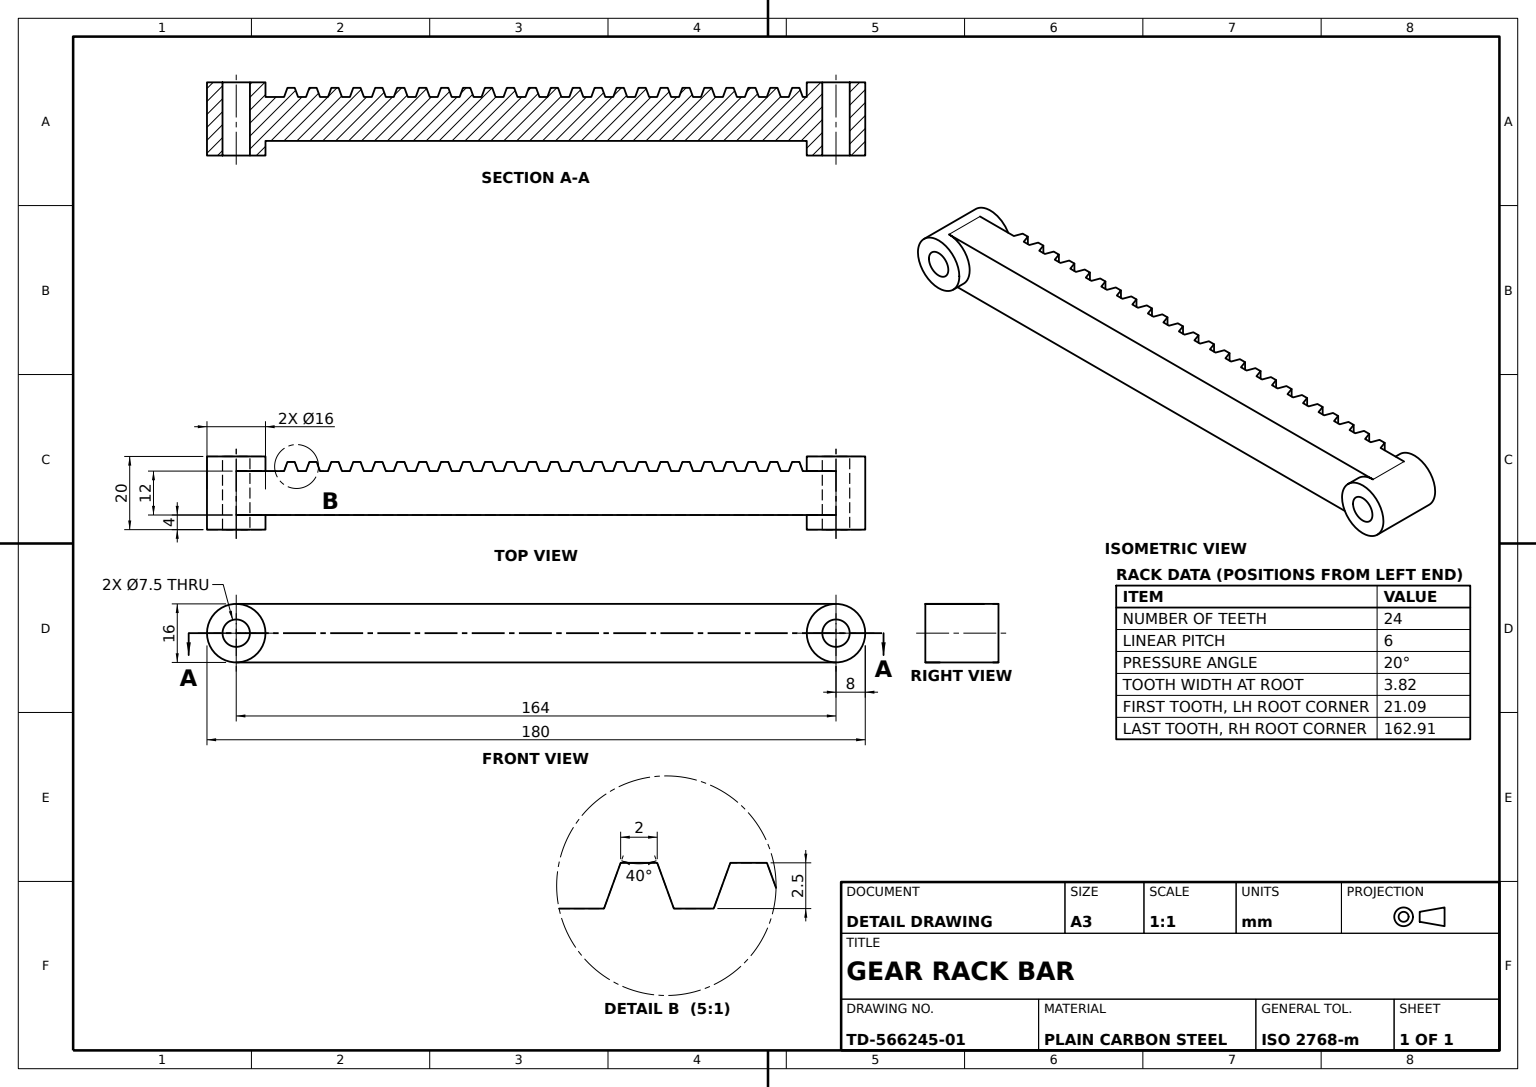
SolidWorks part; units mm, degrees
material "Plain Carbon Steel"
ref_plane "Front Plane" through (0, 0, 0) normal (0, 0, 1) x (1, 0, 0)
ref_plane "Top Plane" through (0, 0, 0) normal (0, 1, 0) x (1, 0, 0)
ref_plane "Right Plane" through (0, 0, 0) normal (1, 0, 0) x (0, 0, -1)
sketch "Eye Bar Profile Sketch" plane through (0, 0, 0) normal (1, 0, 0) x (0, 0, -1)
  circle A0 centre (0, 0) radius 8
  circle A1 centre (0, 0) radius 3.75
  circle A2 centre (-164, 0) radius 8
  circle A3 centre (-164, 0) radius 3.75
  dimension "D1" = 7.5
  dimension "D2" = 7.5
  dimension "D3" = 16
  dimension "D4" = 16
  dimension "D5" = 164
extrude "Bar With Eye Ends" add sketch "Eye Bar Profile Sketch" along normal mid plane 20
sketch "Rack Body Sketch" plane through (0, 0, 0) normal (1, 0, 0) x (0, 0, -1)
  line L1 (-164, 8) -> (0, 8)
  line L3 (-164, -8) -> (0, -8)
  circle A0 centre (-164, 0) radius 8 construction
  circle A1 centre (0, 0) radius 8 construction
  arc A2 (-164, -8) -> (-164, 8) centre (-164, 0) ccw
  circle A3 centre (0, 0) radius 8
  arc A4 (0, 8) -> (0, -8) centre (0, 0) ccw
  dimension "D1" = 0
extrude "Rack Body" add sketch "Rack Body Sketch" along normal mid plane 12
sketch "Rack Teeth Profile Sketch" plane through (0, 0, 0) normal (0, 1, 0) x (1, 0, 0)
  line L0 (0, 0) -> (-8.5, 0) construction
  line L1 (-10, 8) -> (-10, -10) construction
  line L2 (-8.5, 0) -> (-8.5, -10) construction
  line L3 (-8.5, -10) -> (-8.5, -12)
  line L4 (-8.5, -11) -> (-6, -11) construction
  line L5 (-6, 0) -> (-6, -164) construction
  line L6 (-8.5, -10) -> (-5.4907, -8.9047)
  line L7 (-8.5, -12) -> (-5.4907, -13.0953)
  line L8 (-5.4907, -8.9047) -> (-5.4907, -13.0953)
  line L9 (-8.5, -16) -> (-5.4907, -14.9047)
  line L10 (-5.4907, -14.9047) -> (-5.4907, -19.0953)
  line L11 (-8.5, -18) -> (-5.4907, -19.0953)
  line L12 (-8.5, -16) -> (-8.5, -18)
  line L13 (-8.5, -22) -> (-5.4907, -20.9047)
  line L14 (-5.4907, -20.9047) -> (-5.4907, -25.0953)
  line L15 (-8.5, -24) -> (-5.4907, -25.0953)
  line L16 (-8.5, -22) -> (-8.5, -24)
  line L17 (-8.5, -28) -> (-5.4907, -26.9047)
  line L18 (-5.4907, -26.9047) -> (-5.4907, -31.0953)
  line L19 (-8.5, -30) -> (-5.4907, -31.0953)
  line L20 (-8.5, -28) -> (-8.5, -30)
  line L21 (-8.5, -34) -> (-5.4907, -32.9047)
  line L22 (-5.4907, -32.9047) -> (-5.4907, -37.0953)
  line L23 (-8.5, -36) -> (-5.4907, -37.0953)
  line L24 (-8.5, -34) -> (-8.5, -36)
  line L25 (-8.5, -40) -> (-5.4907, -38.9047)
  line L26 (-5.4907, -38.9047) -> (-5.4907, -43.0953)
  line L27 (-8.5, -42) -> (-5.4907, -43.0953)
  line L28 (-8.5, -40) -> (-8.5, -42)
  line L29 (-8.5, -46) -> (-5.4907, -44.9047)
  line L30 (-5.4907, -44.9047) -> (-5.4907, -49.0953)
  line L31 (-8.5, -48) -> (-5.4907, -49.0953)
  line L32 (-8.5, -46) -> (-8.5, -48)
  line L33 (-8.5, -52) -> (-5.4907, -50.9047)
  line L34 (-5.4907, -50.9047) -> (-5.4907, -55.0953)
  line L35 (-8.5, -54) -> (-5.4907, -55.0953)
  line L36 (-8.5, -52) -> (-8.5, -54)
  line L37 (-8.5, -58) -> (-5.4907, -56.9047)
  line L38 (-5.4907, -56.9047) -> (-5.4907, -61.0953)
  line L39 (-8.5, -60) -> (-5.4907, -61.0953)
  line L40 (-8.5, -58) -> (-8.5, -60)
  line L41 (-8.5, -64) -> (-5.4907, -62.9047)
  line L42 (-5.4907, -62.9047) -> (-5.4907, -67.0953)
  line L43 (-8.5, -66) -> (-5.4907, -67.0953)
  line L44 (-8.5, -64) -> (-8.5, -66)
  line L45 (-8.5, -70) -> (-5.4907, -68.9047)
  line L46 (-5.4907, -68.9047) -> (-5.4907, -73.0953)
  line L47 (-8.5, -72) -> (-5.4907, -73.0953)
  line L48 (-8.5, -70) -> (-8.5, -72)
  line L49 (-8.5, -76) -> (-5.4907, -74.9047)
  line L50 (-5.4907, -74.9047) -> (-5.4907, -79.0953)
  line L51 (-8.5, -78) -> (-5.4907, -79.0953)
  line L52 (-8.5, -76) -> (-8.5, -78)
  line L53 (-8.5, -82) -> (-5.4907, -80.9047)
  line L54 (-5.4907, -80.9047) -> (-5.4907, -85.0953)
  line L55 (-8.5, -84) -> (-5.4907, -85.0953)
  line L56 (-8.5, -82) -> (-8.5, -84)
  line L57 (-8.5, -88) -> (-5.4907, -86.9047)
  line L58 (-5.4907, -86.9047) -> (-5.4907, -91.0953)
  line L59 (-8.5, -90) -> (-5.4907, -91.0953)
  line L60 (-8.5, -88) -> (-8.5, -90)
  line L61 (-8.5, -94) -> (-5.4907, -92.9047)
  line L62 (-5.4907, -92.9047) -> (-5.4907, -97.0953)
  line L63 (-8.5, -96) -> (-5.4907, -97.0953)
  line L64 (-8.5, -94) -> (-8.5, -96)
  line L65 (-8.5, -100) -> (-5.4907, -98.9047)
  line L66 (-5.4907, -98.9047) -> (-5.4907, -103.0953)
  line L67 (-8.5, -102) -> (-5.4907, -103.0953)
  line L68 (-8.5, -100) -> (-8.5, -102)
  line L69 (-8.5, -106) -> (-5.4907, -104.9047)
  line L70 (-5.4907, -104.9047) -> (-5.4907, -109.0953)
  line L71 (-8.5, -108) -> (-5.4907, -109.0953)
  line L72 (-8.5, -106) -> (-8.5, -108)
  line L73 (-8.5, -112) -> (-5.4907, -110.9047)
  line L74 (-5.4907, -110.9047) -> (-5.4907, -115.0953)
  line L75 (-8.5, -114) -> (-5.4907, -115.0953)
  line L76 (-8.5, -112) -> (-8.5, -114)
  line L77 (-8.5, -118) -> (-5.4907, -116.9047)
  line L78 (-5.4907, -116.9047) -> (-5.4907, -121.0953)
  line L79 (-8.5, -120) -> (-5.4907, -121.0953)
  line L80 (-8.5, -118) -> (-8.5, -120)
  line L81 (-8.5, -124) -> (-5.4907, -122.9047)
  line L82 (-5.4907, -122.9047) -> (-5.4907, -127.0953)
  line L83 (-8.5, -126) -> (-5.4907, -127.0953)
  line L84 (-8.5, -124) -> (-8.5, -126)
  line L85 (-8.5, -130) -> (-5.4907, -128.9047)
  line L86 (-5.4907, -128.9047) -> (-5.4907, -133.0953)
  line L87 (-8.5, -132) -> (-5.4907, -133.0953)
  line L88 (-8.5, -130) -> (-8.5, -132)
  line L89 (-8.5, -136) -> (-5.4907, -134.9047)
  line L90 (-5.4907, -134.9047) -> (-5.4907, -139.0953)
  line L91 (-8.5, -138) -> (-5.4907, -139.0953)
  line L92 (-8.5, -136) -> (-8.5, -138)
  line L93 (-8.5, -142) -> (-5.4907, -140.9047)
  line L94 (-5.4907, -140.9047) -> (-5.4907, -145.0953)
  line L95 (-8.5, -144) -> (-5.4907, -145.0953)
  line L96 (-8.5, -142) -> (-8.5, -144)
  line L97 (-8.5, -148) -> (-5.4907, -146.9047)
  line L98 (-5.4907, -146.9047) -> (-5.4907, -151.0953)
  line L99 (-8.5, -150) -> (-5.4907, -151.0953)
  line L100 (-8.5, -148) -> (-8.5, -150)
  dimension "D1" = 8.5
  dimension "D2" = 18
  dimension "D3" = 2
  dimension "D4" = 20
  dimension "D5" = 18
  dimension "D7" = 4.5093
  dimension "D8" = 14.9047
  dimension "D6" = 24
extrude "Rack Teeth 24x" add sketch "Rack Teeth Profile Sketch" along normal mid plane 16
